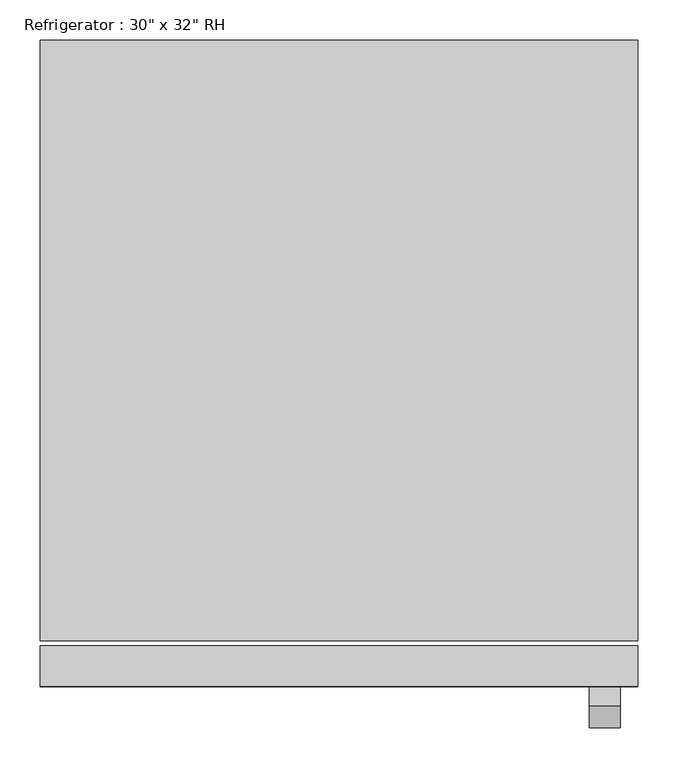
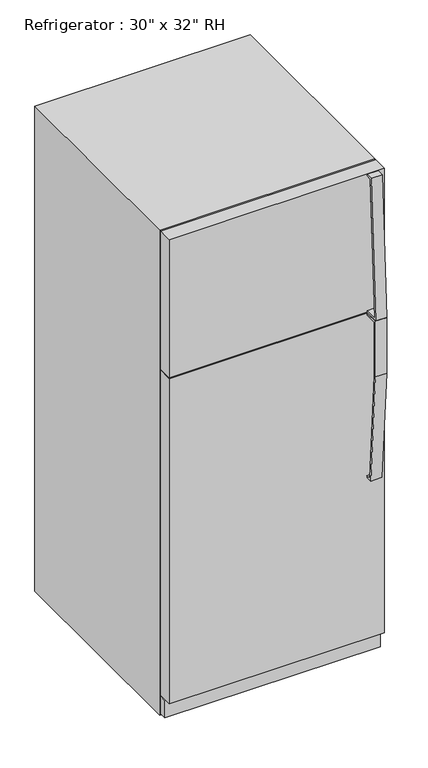
"""IFC4 building model written with IfcOpenShell, lengths in millimetres: proxy geometry."""

from ifc_helpers import new_model, si_unit, frame, origin, origin_with_axes, place, context, project, spatial, polyline, outline, extrude, source, transform, mapped, element, save


def proxy_a13a33b2(model_context):
    return source(origin(), model_context, "Body", "SweptSolid", [
        extrude(outline(polyline([(-417.9010285, 1262.0625), (-462.3510285, 1262.0625), (-462.3510285, 1065.4342469), (-434.8723987, 672.4715334), (-417.9010285, 672.4715334), (-417.9010285, 666.1370017), (-440.7949512, 666.1370017), (-468.7010285, 1065.2125), (-468.7010285, 1268.4125), (-417.9010285, 1268.4125), (-417.9010285, 1262.0625)])), frame((312.7375, 0.0, 0.0), z_axis=(1.0, 0.0, 0.0), x_axis=(0.0, 1.0, 0.0)), (0.0, 0.0, 1.0), 38.4332978),
        extrude(outline(polyline([(-442.739413, 1778.0), (-418.6780855, 1778.0), (-418.6780855, 1771.65), (-437.5263449, 1771.65), (-463.4007207, 1277.9375), (-418.6780855, 1277.9375), (-418.6780855, 1271.5875), (-469.2793675, 1271.5875), (-442.739413, 1778.0)])), frame((312.7375, 0.0, 0.0), z_axis=(1.0, 0.0, 0.0), x_axis=(0.0, 1.0, 0.0)), (0.0, 0.0, 1.0), 38.4332978),
        extrude(outline(polyline([(373.0625, -367.1010285), (373.0625, -392.5010285), (-373.0625, -392.5010285), (-373.0625, -367.1010285), (373.0625, -367.1010285)])), frame((0.0, 0.0, 9.3816357), z_axis=(0.0, 0.0, 1.0), x_axis=(1.0, 0.0, 0.0)), (0.0, 0.0, 1.0), 63.5),
        extrude(outline(polyline([(373.0625, -367.1010285), (373.0625, -417.9010285), (-373.0625, -417.9010285), (-373.0625, -367.1010285), (373.0625, -367.1010285)])), frame((0.0, 0.0, 76.2), z_axis=(0.0, 0.0, 1.0), x_axis=(1.0, 0.0, 0.0)), (0.0, 0.0, 1.0), 1192.2125),
        extrude(outline(polyline([(373.0625, -367.1010285), (373.0625, -417.9010285), (-373.0625, -417.9010285), (-373.0625, -367.1010285), (373.0625, -367.1010285)])), frame((0.0, 0.0, 1271.5875), z_axis=(0.0, 0.0, 1.0), x_axis=(1.0, 0.0, 0.0)), (0.0, 0.0, 1.0), 506.4125),
        extrude(outline(polyline([(373.0625, 388.5489715), (373.0625, -360.7510285), (-373.0625, -360.7510285), (-373.0625, 388.5489715), (373.0625, 388.5489715)])), origin_with_axes(), (0.0, 0.0, 1.0), 1778.0),
    ])


if __name__ == "__main__":
    model = new_model("IFC4")
    model_context = context("Model", 3, world=origin())
    ifc_project = project(units=[si_unit("LENGTHUNIT", "METRE", prefix="MILLI")], contexts=[model_context])
    site = spatial("IfcSite", under=ifc_project)
    building = spatial("IfcBuilding", under=site)
    placement = place(None, origin())
    proxy_shape = proxy_a13a33b2(model_context)
    element("IfcBuildingElementProxy", 1, Name="Refrigerator : 30\" x 32\" RH", ObjectType="Refrigerator : 30\" x 32\" RH", at=placement, inside=building, context=model_context, shape_type="MappedRepresentation", body=[
        mapped(proxy_shape, transform((0.0, 0.0, 0.0), x_axis=(1.0, 0.0, 0.0), y_axis=(0.0, 1.0, 0.0), z_axis=(0.0, 0.0, 1.0))),
    ])
    save(model, "model.ifc")

# Revit data of these elements
# Type "Refrigerator : 30\" x 32\" RH"
#   Label = "REF."
#   Assembly Code = "E1090400"
#   Depth = 2' - 7 3/4"
#   Handle = 2' - 3"
#   Height = 5' - 10"
#   Rear Clearance = 0' - 2"
#   Top Door Height = 1' - 8"
#   Width = 2' - 5 3/8"
#   Material = Cherry
#   Default Elevation = 0
# Element 1 (IfcBuildingElementProxy, "Refrigerator : 30\" x 32\" RH")
#   Materials on its faces: "Cherry", "Steel, Chrome Plated"
# Materials
#   "Cherry": class "Wood", colour RGB 226 177 128, transparency 0, Description = "Prunus Serotina", Cost = 0
#   "Steel, Chrome Plated": class "Metal", colour RGB 17 17 17, transparency 0, Description = "Chromiuim plated steel", Cost = 0
